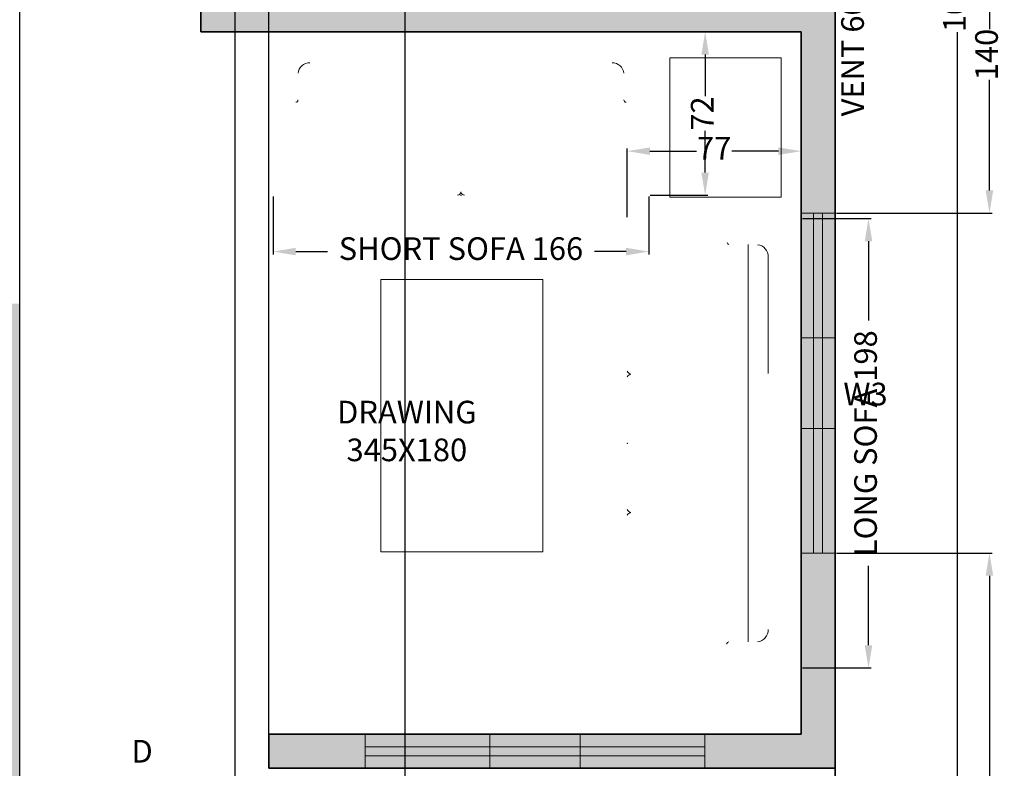
# Model space of a CAD drawing. Units: centimetres. Extents: x 2401 to 3632, y 2122 to 3526.
# Tile 6 of 10: x 2885 to 3320, y 2591 to 2921. Entities that reach past the tile are written whole.
import ezdxf

# ---------------------------------------------------------------- set-up
doc = ezdxf.new("R2010")
doc.units = ezdxf.units.CM
for name, color, linetype, lineweight in [('A-ANNO-DIMS', 9, 'Continuous', 18), ('A-ANNO-TEXT', 9, 'Continuous', 18), ('A-AREA-IDEN', 9, 'Continuous', 25), ('A-FURN', 9, 'Continuous', 18), ('A-GLAZ', 4, 'Continuous', 18), ('A-WALL', 7, 'Continuous', 35)]:
    doc.layers.add(name, color=color, linetype=linetype, lineweight=lineweight)
doc.layers.add('A-GLAZ-PATT', color=251, linetype='Continuous', lineweight=13, true_color=0x636466)
doc.layers.add('A-WALL-PATT', color=18, linetype='Continuous', lineweight=13, true_color=0x000000)
doc.styles.get("Standard").update_dxf_attribs({"font": 'arial.ttf'})
doc.dimstyles.new('ISO-25', dxfattribs={"dimtxt": 10, "dimasz": 10, "dimexe": 1.25, "dimexo": 0.625, "dimtad": 0, "dimtxsty": 'Standard', "dimcen": 2.5, "dimadec": 0, "dimazin": 0, "dimtfac": 1, "dimtmove": 0, "dimatfit": 3, "dimfxl": 1, "dimarcsym": 0})

# ---------------------------------------------------------------- blocks, each defined once
blk = doc.blocks.new('Clinicians and patient chairs 9_dwgmodels.com')
at = {"color": 0}
for points in [[(-907.9, 0, 0, 0, 0), (-959.6, -11.1, 4.62, 4.62, 0)], [(907.9, 0, 0, 0, 0), (-907.9, 0, 4.62, 4.62, 0)], [(959.6, -11.1, 0, 0, 0), (907.9, 0, 4.62, 4.62, 0)], [(-994.7, -35.9, 0, 0, 0), (-1015.6, -68.3, 4.62, 4.62, 0)], [(-959.6, -11.1, 0, 0, 0), (-994.7, -35.9, 4.62, 4.62, 0)], [(994.7, -35.9, 0, 0, 0), (959.6, -11.1, 4.62, 4.62, 0)], [(1015.6, -68.3, 0, 0, 0), (994.7, -35.9, 4.62, 4.62, 0)], [(-1015.6, -68.3, 0, 0, 0), (-1025.5, -106.3, 4.62, 4.62, 0)], [(1025.5, -106.3, 0, 0, 0), (1015.6, -68.3, 4.62, 4.62, 0)], [(-1025.5, -106.3, 0, 0, 0), (-1025.5, -779.5, 4.62, 4.62, 0)], [(1025.5, -779.5, 0, 0, 0), (1025.5, -106.3, 4.62, 4.62, 0)], [(1025.5, -779.5, 0, 0, 0), (1025.5, -117.3, 4.62, 4.62, 0)], [(-313.4, -149.9, 0, 0, 0), (-318.1, -149.9, 4.62, 4.62, 0)], [(-314.5, -150.4, 0, 0, 0), (-315.7, -159.3, 4.62, 4.62, 0)], [(-315.7, -159.3, 0, 0, 0), (-315.7, -777.3, 4.62, 4.62, 0)], [(-309.5, -148.3, 0, 0, 0), (-314.5, -150.4, 4.62, 4.62, 0)], [(-308, -148.3, 0, 0, 0), (-309.5, -148.3, 4.62, 4.62, 0)], [(-307.5, -148.3, 0, 0, 0), (-308, -148.3, 4.62, 4.62, 0)], [(242.9, -148.3, 0, 0, 0), (-307.5, -148.3, 4.62, 4.62, 0)], [(242.9, -148.3, 0, 0, 0), (296, -148.3, 4.62, 4.62, 0)], [(296, -148.3, 0, 0, 0), (307.5, -148.3, 4.62, 4.62, 0)], [(308, -148.3, 0, 0, 0), (307.5, -148.3, 4.62, 4.62, 0)], [(309.5, -148.3, 0, 0, 0), (308, -148.3, 4.62, 4.62, 0)], [(309.5, -148.3, 0, 0, 0), (314.5, -150.4, 4.62, 4.62, 0)], [(849.5, -149.9, 0, 0, 0), (313.4, -149.9, 4.62, 4.62, 0)], [(314.5, -150.4, 0, 0, 0), (315.7, -159.3, 4.62, 4.62, 0)], [(315.7, -159.3, 0, 0, 0), (315.7, -777.3, 4.62, 4.62, 0)], [(315.7, -161.8, 0, 0, 0), (315.7, -777.3, 4.62, 4.62, 0)], [(-906.6, -285, 0, 0, 0), (-906.4, -198.1, 4.62, 4.62, 0)], [(906.9, -327, 0, 0, 0), (906.4, -199.7, 4.62, 4.62, 0)], [(-906.8, -305.4, 0, 0, 0), (-906.9, -324.5, 4.62, 4.62, 0)], [(-906.6, -285, 0, 0, 0), (-906.8, -305.4, 4.62, 4.62, 0)], [(-1023, -329.7, 0, 0, 0), (-1019.2, -332.9, 4.62, 4.62, 0)], [(-1019.8, -340.2, 0, 0, 0), (-1023, -348.6, 4.62, 4.62, 0)], [(-1010.3, -335.9, 0, 0, 0), (-1019.8, -340.2, 4.62, 4.62, 0)], [(-1019.2, -332.9, 0, 0, 0), (-1019, -333, 4.62, 4.62, 0)], [(-1019, -333, 0, 0, 0), (-1018.9, -333.1, 4.62, 4.62, 0)], [(-1013.9, -334.2, 0, 0, 0), (-1018.9, -333.1, 4.62, 4.62, 0)], [(-1013.9, -334.2, 0, 0, 0), (-964.4, -335.7, 4.62, 4.62, 0)], [(-917.1, -337, 0, 0, 0), (-1010.3, -335.9, 4.62, 4.62, 0)], [(-964.4, -335.7, 0, 0, 0), (-927.1, -336.8, 4.62, 4.62, 0)], [(-906.9, -324.5, 0, 0, 0), (-906.9, -329.8, 4.62, 4.62, 0)], [(906.9, -327, 0, 0, 0), (906.9, -329.9, 4.62, 4.62, 0)], [(964.4, -335.7, 0, 0, 0), (914.9, -337.2, 4.62, 4.62, 0)], [(917.1, -339.4, 0, 0, 0), (1010.3, -338.4, 4.62, 4.62, 0)], [(1013.9, -334.2, 0, 0, 0), (964.4, -335.7, 4.62, 4.62, 0)], [(1010.3, -338.4, 0, 0, 0), (1019.8, -342.7, 4.62, 4.62, 0)], [(1013.9, -334.2, 0, 0, 0), (1018.9, -333.1, 4.62, 4.62, 0)], [(1018.9, -333.1, 0, 0, 0), (1019, -333, 4.62, 4.62, 0)], [(1019.2, -332.9, 0, 0, 0), (1019, -333, 4.62, 4.62, 0)], [(1023, -329.7, 0, 0, 0), (1019.2, -332.9, 4.62, 4.62, 0)], [(1019.8, -342.7, 0, 0, 0), (1023, -351.1, 4.62, 4.62, 0)], [(1023, -351.1, 0, 0, 0), (1022.6, -779.8, 4.62, 4.62, 0)], [(-1025.5, -779.5, 0, 0, 0), (-1022.2, -788.7, 4.62, 4.62, 0)], [(-1022.2, -788.7, 0, 0, 0), (-1021.6, -789.8, 4.62, 4.62, 0)], [(-1021.6, -789.8, 0, 0, 0), (-1020.6, -790.5, 4.62, 4.62, 0)], [(-1020.6, -790.5, 0, 0, 0), (-1013.6, -793.7, 4.62, 4.62, 0)], [(-1013.6, -793.7, 0, 0, 0), (1013.6, -793.7, 4.62, 4.62, 0)], [(1019.8, -788.8, 0, 0, 0), (1013.1, -793.7, 4.62, 4.62, 0)], [(1013.6, -793.7, 0, 0, 0), (1020.6, -790.5, 4.62, 4.62, 0)], [(1022.6, -779.8, 0, 0, 0), (1019.8, -788.8, 4.62, 4.62, 0)], [(1020.6, -790.5, 0, 0, 0), (1021.6, -789.8, 4.62, 4.62, 0)], [(1022.2, -788.7, 0, 0, 0), (1021.6, -789.8, 4.62, 4.62, 0)], [(1022.2, -788.7, 0, 0, 0), (1025.5, -779.5, 4.62, 4.62, 0)]]:
    blk.add_lwpolyline(points, format="xyseb", dxfattribs=at)
for points in [[(-849.5, -149.9), (-318.1, -149.9)], [(-906.5, -241.5), (906.5, -242.3)]]:
    blk.add_lwpolyline(points, dxfattribs=at)
for centre, radius, start, end in [((-851.7, -204.8), 54.9, 87.6679, 174.7256), ((851.7, -204.8), 54.9, 5.2744, 92.3321), ((-916.6, -326.8), 10.2, 267.5454, 342.4057), ((916.9, -329.4), 10, 182.6094, 270.795), ((-337, -773.8), 21.5, 292.115, 350.6304), ((-294.5, -773.8), 21.5, 189.3696, 247.885), ((294.5, -773.8), 21.5, 292.115, 350.6304), ((336.9, -773.8), 21.5, 189.3696, 247.885)]:
    blk.add_arc(centre, radius, start, end, dxfattribs=at)
blk.add_point((0, -793.7), dxfattribs=at)
blk = doc.blocks.new('Clinicians and patient chairs 13_dwgmodels.com')
at = {"color": 0}
for points in [[(-780.9, 0, 0, 0, 0), (-832.6, -11.1, 4.5, 4.5, 0)], [(-780.8, -0.7, 0, 0, 0), (-832.3, -11.8, 4.5, 4.5, 0)], [(-780.8, -0.7, 0, 0, 0), (-832.3, -11.8, 4.5, 4.5, 0)], [(780.9, 0, 0, 0, 0), (-780.9, 0, 4.5, 4.5, 0)], [(780.8, -0.7, 0, 0, 0), (-780.8, -0.7, 4.5, 4.5, 0)], [(780.8, -0.7, 0, 0, 0), (-780.8, -0.7, 4.5, 4.5, 0)], [(832.3, -11.8, 0, 0, 0), (780.8, -0.7, 4.5, 4.5, 0)], [(832.3, -11.8, 0, 0, 0), (780.8, -0.7, 4.5, 4.5, 0)], [(832.6, -11.1, 0, 0, 0), (780.9, 0, 4.5, 4.5, 0)], [(-867.7, -35.9, 0, 0, 0), (-888.6, -68.3, 4.5, 4.5, 0)], [(-867.1, -36.4, 0, 0, 0), (-888, -68.6, 4.5, 4.5, 0)], [(-867.1, -36.4, 0, 0, 0), (-888, -68.6, 4.5, 4.5, 0)], [(-872.1, -47.4, 0, 0, 0), (-872.1, -47.3, 4.5, 4.5, 0)], [(-832.6, -11.1, 0, 0, 0), (-867.7, -35.9, 4.5, 4.5, 0)], [(-832.3, -11.8, 0, 0, 0), (-867.1, -36.4, 4.5, 4.5, 0)], [(-832.3, -11.8, 0, 0, 0), (-867.1, -36.4, 4.5, 4.5, 0)], [(-854.1, -29.4, 0, 0, 0), (-854.1, -29.4, 4.5, 4.5, 0)], [(867.1, -36.4, 0, 0, 0), (832.3, -11.8, 4.5, 4.5, 0)], [(867.1, -36.4, 0, 0, 0), (832.3, -11.8, 4.5, 4.5, 0)], [(867.7, -35.9, 0, 0, 0), (832.6, -11.1, 4.5, 4.5, 0)], [(888, -68.6, 0, 0, 0), (867.1, -36.4, 4.5, 4.5, 0)], [(888, -68.6, 0, 0, 0), (867.1, -36.4, 4.5, 4.5, 0)], [(888.6, -68.3, 0, 0, 0), (867.7, -35.9, 4.5, 4.5, 0)], [(-888.6, -68.3, 0, 0, 0), (-898.5, -106.3, 4.5, 4.5, 0)], [(-888, -68.6, 0, 0, 0), (-897.8, -106.4, 4.5, 4.5, 0)], [(897.8, -106.4, 0, 0, 0), (888, -68.6, 4.5, 4.5, 0)], [(897.8, -106.4, 0, 0, 0), (888, -68.6, 4.5, 4.5, 0)], [(898.5, -106.3, 0, 0, 0), (888.6, -68.3, 4.5, 4.5, 0)], [(-898.5, -106.3, 0, 0, 0), (-898.5, -766.8, 4.5, 4.5, 0)], [(-897.8, -106.4, 0, 0, 0), (-897.8, -114.4, 4.5, 4.5, 0)], [(-897.8, -106.4, 0, 0, 0), (-897.8, -114.4, 4.5, 4.5, 0)], [(-897.8, -114.4, 0, 0, 0), (-897.8, -766.7, 4.5, 4.5, 0)], [(-897.8, -114.4, 0, 0, 0), (-897.8, -766.7, 4.5, 4.5, 0)], [(-897.8, -766.7, 0, 0, 0), (-897.8, -114.4, 4.5, 4.5, 0)], [(-896, -117.6, 0, 0, 0), (-896, -126.8, 4.5, 4.5, 0)], [(-896, -117.6, 0, 0, 0), (-896, -324.6, 4.5, 4.5, 0)], [(-896, -126.8, 0, 0, 0), (-896, -324.6, 4.5, 4.5, 0)], [(897.8, -114.4, 0, 0, 0), (897.8, -106.4, 4.5, 4.5, 0)], [(897.8, -114.4, 0, 0, 0), (897.8, -106.4, 4.5, 4.5, 0)], [(897.8, -766.7, 0, 0, 0), (897.8, -114.4, 4.5, 4.5, 0)], [(898.5, -766.8, 0, 0, 0), (898.5, -106.3, 4.5, 4.5, 0)], [(898.5, -766.8, 0, 0, 0), (898.5, -117.3, 4.5, 4.5, 0)], [(-22.2, -148.3, 0, 0, 0), (-722.5, -148.3, 4.5, 4.5, 0)], [(-8.3, -148.3, 0, 0, 0), (-22.2, -148.3, 4.5, 4.5, 0)], [(-8.3, -148.3, 0, 0, 0), (-7.7, -148.3, 4.5, 4.5, 0)], [(-7.7, -148.3, 0, 0, 0), (-6.2, -148.3, 4.5, 4.5, 0)], [(-6.2, -148.3, 0, 0, 0), (-1.3, -150.4, 4.5, 4.5, 0)], [(2.3, -149.9, 0, 0, 0), (-2.3, -149.9, 4.5, 4.5, 0)], [(-1.3, -150.4, 0, 0, 0), (0, -159.3, 4.5, 4.5, 0)], [(1.3, -150.4, 0, 0, 0), (0, -159.3, 4.5, 4.5, 0)], [(0, -159.3, 0, 0, 0), (0, -764.6, 4.5, 4.5, 0)], [(0, -159.3, 0, 0, 0), (0, -764.6, 4.5, 4.5, 0)], [(6.2, -148.3, 0, 0, 0), (1.3, -150.4, 4.5, 4.5, 0)], [(7.7, -148.3, 0, 0, 0), (6.2, -148.3, 4.5, 4.5, 0)], [(8.3, -148.3, 0, 0, 0), (7.7, -148.3, 4.5, 4.5, 0)], [(22.2, -148.3, 0, 0, 0), (8.3, -148.3, 4.5, 4.5, 0)], [(206.6, -148.3, 0, 0, 0), (22.2, -148.3, 4.5, 4.5, 0)], [(206.6, -148.3, 0, 0, 0), (722.5, -148.3, 4.5, 4.5, 0)], [(-779.6, -285, 0, 0, 0), (-779.4, -198.1, 4.5, 4.5, 0)], [(779.6, -285, 0, 0, 0), (779.4, -198.1, 4.5, 4.5, 0)], [(-896, -321.9, 0, 0, 0), (-896, -251.5, 4.5, 4.5, 0)], [(-896, -317.7, 0, 0, 0), (-896, -329.7, 4.5, 4.5, 0)], [(-896, -320.4, 0, 0, 0), (-896, -324.6, 4.5, 4.5, 0)], [(-896, -321.9, 0, 0, 0), (-896, -329.7, 4.5, 4.5, 0)], [(-896, -329.7, 0, 0, 0), (-896, -321.9, 4.5, 4.5, 0)], [(-896, -329.7, 0, 0, 0), (-892.2, -332.9, 4.5, 4.5, 0)], [(-779.8, -305.4, 0, 0, 0), (-779.9, -324.5, 4.5, 4.5, 0)], [(-779.6, -285, 0, 0, 0), (-779.8, -305.4, 4.5, 4.5, 0)], [(779.6, -285, 0, 0, 0), (779.8, -305.4, 4.5, 4.5, 0)], [(779.8, -305.4, 0, 0, 0), (779.9, -324.5, 4.5, 4.5, 0)], [(896, -329.7, 0, 0, 0), (892.2, -332.9, 4.5, 4.5, 0)], [(-892.2, -332.9, 0, 0, 0), (-892, -333, 4.5, 4.5, 0)], [(-892, -333, 0, 0, 0), (-891.9, -333.1, 4.5, 4.5, 0)], [(-886.9, -334.2, 0, 0, 0), (-891.9, -333.1, 4.5, 4.5, 0)], [(-886.9, -334.2, 0, 0, 0), (-837.4, -335.7, 4.5, 4.5, 0)], [(-837.4, -335.7, 0, 0, 0), (-790.1, -337, 4.5, 4.5, 0)], [(837.4, -335.7, 0, 0, 0), (790.1, -337, 4.5, 4.5, 0)], [(886.9, -334.2, 0, 0, 0), (837.4, -335.7, 4.5, 4.5, 0)], [(886.9, -334.2, 0, 0, 0), (891.9, -333.1, 4.5, 4.5, 0)], [(891.9, -333.1, 0, 0, 0), (892, -333, 4.5, 4.5, 0)], [(892.2, -332.9, 0, 0, 0), (892, -333, 4.5, 4.5, 0)], [(-898.5, -766.8, 0, 0, 0), (-895.2, -776, 4.5, 4.5, 0)], [(-895.2, -776, 0, 0, 0), (-898.5, -766.8, 4.5, 4.5, 0)], [(-897.8, -766.7, 0, 0, 0), (-894.5, -775.7, 4.5, 4.5, 0)], [(-897.8, -766.7, 0, 0, 0), (-894.5, -775.7, 4.5, 4.5, 0)], [(-894.5, -775.7, 0, 0, 0), (-897.8, -766.7, 4.5, 4.5, 0)], [(-894.5, -775.7, 0, 0, 0), (-897.8, -766.7, 4.5, 4.5, 0)], [(-895.2, -776, 0, 0, 0), (-894.6, -777.1, 4.5, 4.5, 0)], [(-894.6, -777.1, 0, 0, 0), (-895.2, -776, 4.5, 4.5, 0)], [(-894.5, -775.7, 0, 0, 0), (-894, -776.6, 4.5, 4.5, 0)], [(-894.5, -775.7, 0, 0, 0), (-894, -776.6, 4.5, 4.5, 0)], [(-894, -776.6, 0, 0, 0), (-894.5, -775.7, 4.5, 4.5, 0)], [(-894, -776.6, 0, 0, 0), (-894.5, -775.7, 4.5, 4.5, 0)], [(-894.6, -777.1, 0, 0, 0), (-893.6, -777.8, 4.5, 4.5, 0)], [(-893.6, -777.8, 0, 0, 0), (-894.6, -777.1, 4.5, 4.5, 0)], [(-894, -776.6, 0, 0, 0), (-893.2, -777.2, 4.5, 4.5, 0)], [(-894, -776.6, 0, 0, 0), (-893.2, -777.2, 4.5, 4.5, 0)], [(-893.2, -777.2, 0, 0, 0), (-894, -776.6, 4.5, 4.5, 0)], [(-893.2, -777.2, 0, 0, 0), (-894, -776.6, 4.5, 4.5, 0)], [(-893.6, -777.8, 0, 0, 0), (-886.6, -781, 4.5, 4.5, 0)], [(-886.6, -781, 0, 0, 0), (-893.6, -777.8, 4.5, 4.5, 0)], [(-893.2, -777.2, 0, 0, 0), (-886.5, -780.3, 4.5, 4.5, 0)], [(-893.2, -777.2, 0, 0, 0), (-886.5, -780.3, 4.5, 4.5, 0)], [(-886.5, -780.3, 0, 0, 0), (-893.2, -777.2, 4.5, 4.5, 0)], [(-886.5, -780.3, 0, 0, 0), (-893.2, -777.2, 4.5, 4.5, 0)], [(-886.6, -781, 0, 0, 0), (886.6, -781, 4.5, 4.5, 0)], [(886.6, -781, 0, 0, 0), (-886.6, -781, 4.5, 4.5, 0)], [(-886.5, -780.3, 0, 0, 0), (886.5, -780.3, 4.5, 4.5, 0)], [(-886.5, -780.3, 0, 0, 0), (886.5, -780.3, 4.5, 4.5, 0)], [(886.5, -780.3, 0, 0, 0), (-886.5, -780.3, 4.5, 4.5, 0)], [(886.5, -780.3, 0, 0, 0), (-886.5, -780.3, 4.5, 4.5, 0)], [(886.5, -780.3, 0, 0, 0), (893.2, -777.2, 4.5, 4.5, 0)], [(886.5, -780.3, 0, 0, 0), (893.2, -777.2, 4.5, 4.5, 0)], [(893.2, -777.2, 0, 0, 0), (886.5, -780.3, 4.5, 4.5, 0)], [(893.2, -777.2, 0, 0, 0), (886.5, -780.3, 4.5, 4.5, 0)], [(886.6, -781, 0, 0, 0), (893.6, -777.8, 4.5, 4.5, 0)], [(893.6, -777.8, 0, 0, 0), (886.6, -781, 4.5, 4.5, 0)], [(893.2, -777.2, 0, 0, 0), (894, -776.6, 4.5, 4.5, 0)], [(893.2, -777.2, 0, 0, 0), (894, -776.6, 4.5, 4.5, 0)], [(894, -776.6, 0, 0, 0), (893.2, -777.2, 4.5, 4.5, 0)], [(894, -776.6, 0, 0, 0), (893.2, -777.2, 4.5, 4.5, 0)], [(893.6, -777.8, 0, 0, 0), (894.6, -777.1, 4.5, 4.5, 0)], [(894.6, -777.1, 0, 0, 0), (893.6, -777.8, 4.5, 4.5, 0)], [(894.5, -775.7, 0, 0, 0), (894, -776.6, 4.5, 4.5, 0)], [(894.5, -775.7, 0, 0, 0), (894, -776.6, 4.5, 4.5, 0)], [(894.5, -775.7, 0, 0, 0), (894, -776.6, 4.5, 4.5, 0)], [(894.5, -775.7, 0, 0, 0), (894, -776.6, 4.5, 4.5, 0)], [(894.5, -775.7, 0, 0, 0), (897.8, -766.7, 4.5, 4.5, 0)], [(894.5, -775.7, 0, 0, 0), (897.8, -766.7, 4.5, 4.5, 0)], [(897.8, -766.7, 0, 0, 0), (894.5, -775.7, 4.5, 4.5, 0)], [(897.8, -766.7, 0, 0, 0), (894.5, -775.7, 4.5, 4.5, 0)], [(895.2, -776, 0, 0, 0), (894.6, -777.1, 4.5, 4.5, 0)], [(895.2, -776, 0, 0, 0), (894.6, -777.1, 4.5, 4.5, 0)], [(895.2, -776, 0, 0, 0), (898.5, -766.8, 4.5, 4.5, 0)], [(898.5, -766.8, 0, 0, 0), (895.2, -776, 4.5, 4.5, 0)]]:
    blk.add_lwpolyline(points, format="xyseb", dxfattribs=at)
for points in [[(-779.9, -324.5), (-779.9, -328.3)], [(779.9, -324.5), (779.9, -325.8)]]:
    blk.add_lwpolyline(points, dxfattribs=at)
for centre, radius, start, end in [((-724.7, -203.1), 54.9, 87.6679, 174.7255), ((724.7, -203.1), 54.9, 5.2744, 92.3321), ((-789.7, -327.1), 9.9, 267.955, 352.9309), ((791.8, -325.1), 12, 183.2786, 261.4861), ((-17.2, -763), 17.3, 271.1045, 354.6239), ((17.2, -763), 17.3, 185.3761, 268.8955)]:
    blk.add_arc(centre, radius, start, end, dxfattribs=at)
blk.add_point((0, -781), dxfattribs=at)
blk = doc.blocks.new('*D14')
at = {"layer": 'A-ANNO-DIMS', "color": 0, "lineweight": -2, "transparency": 16777216}
for p, q in [((3246.06, 3451.1), (3300.7, 3451.1)), ((3299.45, 3441.1), (3299.45, 2946.17)), ((3299.45, 2421.1), (3299.45, 2916.04)), ((3246.06, 2411.1), (3300.7, 2411.1))]:
    blk.add_line(p, q, dxfattribs=at)
at = {"layer": 'A-ANNO-DIMS', "color": 0, "transparency": 16777216}
for points in [[(3297.79, 3441.1), (3301.12, 3441.1), (3299.45, 3451.1)], [(3297.79, 2421.1), (3301.12, 2421.1), (3299.45, 2411.1)]]:
    blk.add_solid(points, dxfattribs=at)
at = {"layer": 'Defpoints', "color": 0, "transparency": 16777216}
for p in [(3245.44, 3451.1), (3245.44, 2411.1), (3299.45, 2411.1)]:
    blk.add_point(p, dxfattribs=at)
at = {"layer": 'A-ANNO-DIMS', "color": 0, "transparency": 16777216, "insert": (3299.45, 2931.1), "char_height": 10, "attachment_point": 5, "rotation": 90}
blk.add_mtext('1040', dxfattribs=at)
blk = doc.blocks.new('WIN-1500-3P')
for p, q in [((0, 15), (0, 0)), ((55, 15), (55, 0)), ((95, 15), (95, 0)), ((150, 15), (150, 0)), ((0, 9.5), (150, 9.5)), ((0, 5.5), (150, 5.5))]:
    blk.add_line(p, q)
blk = doc.blocks.new('*D22')
at = {"layer": 'A-ANNO-DIMS', "color": 0, "lineweight": -2, "transparency": 16777216}
for p, q in [((3246.06, 3036.1), (3255.69, 3036.1)), ((3254.44, 3026.1), (3254.44, 2986.1)), ((3246.06, 2976.1), (3255.69, 2976.1)), ((3254.44, 2976.1), (3254.44, 2966.1))]:
    blk.add_line(p, q, dxfattribs=at)
at = {"layer": 'A-ANNO-DIMS', "color": 0, "transparency": 16777216}
for points in [[(3252.77, 3026.1), (3256.1, 3026.1), (3254.44, 3036.1)], [(3252.77, 2986.1), (3256.1, 2986.1), (3254.44, 2976.1)]]:
    blk.add_solid(points, dxfattribs=at)
at = {"layer": 'Defpoints', "color": 0, "transparency": 16777216}
for p in [(3245.44, 3036.1), (3245.44, 2976.1), (3254.44, 2976.1)]:
    blk.add_point(p, dxfattribs=at)
at = {"layer": 'A-ANNO-DIMS', "color": 0, "transparency": 16777216, "insert": (3254.44, 2920.31), "char_height": 10, "attachment_point": 5, "rotation": 90}
blk.add_mtext('VENT 60 TYP.', dxfattribs=at)
blk = doc.blocks.new('*D34')
at = {"layer": 'A-ANNO-DIMS', "color": 0, "lineweight": -2, "transparency": 16777216}
for p, q in [((3231.06, 2833.71), (3261.43, 2833.71)), ((3260.18, 2823.71), (3260.18, 2788.71)), ((3260.18, 2645.39), (3260.18, 2680.4)), ((3231.06, 2635.39), (3261.43, 2635.39))]:
    blk.add_line(p, q, dxfattribs=at)
at = {"layer": 'A-ANNO-DIMS', "color": 0, "transparency": 16777216}
for points in [[(3258.52, 2823.71), (3261.85, 2823.71), (3260.18, 2833.71)], [(3258.52, 2645.39), (3261.85, 2645.39), (3260.18, 2635.39)]]:
    blk.add_solid(points, dxfattribs=at)
at = {"layer": 'Defpoints', "color": 0, "transparency": 16777216}
for p in [(3230.44, 2833.71), (3230.44, 2635.39), (3260.18, 2635.39)]:
    blk.add_point(p, dxfattribs=at)
at = {"layer": 'A-ANNO-DIMS', "color": 0, "transparency": 16777216, "insert": (3260.18, 2734.55), "char_height": 10, "attachment_point": 5, "rotation": 90}
blk.add_mtext('LONG SOFA 198', dxfattribs=at)
blk = doc.blocks.new('*D35')
at = {"layer": 'A-ANNO-DIMS', "color": 0, "lineweight": -2, "transparency": 16777216}
for p, q in [((3153.69, 2834.33), (3153.69, 2864.7)), ((3163.69, 2863.45), (3184.32, 2863.45)), ((3220.44, 2863.45), (3199.81, 2863.45)), ((3230.44, 2834.33), (3230.44, 2864.7))]:
    blk.add_line(p, q, dxfattribs=at)
at = {"layer": 'A-ANNO-DIMS', "color": 0, "transparency": 16777216}
for points in [[(3163.69, 2865.12), (3163.69, 2861.79), (3153.69, 2863.45)], [(3220.44, 2865.12), (3220.44, 2861.79), (3230.44, 2863.45)]]:
    blk.add_solid(points, dxfattribs=at)
at = {"layer": 'Defpoints', "color": 0, "transparency": 16777216}
for p in [(3230.44, 2863.45), (3153.69, 2833.71), (3230.44, 2833.71)]:
    blk.add_point(p, dxfattribs=at)
at = {"layer": 'A-ANNO-DIMS', "color": 0, "transparency": 16777216, "insert": (3192.06, 2863.45), "char_height": 10, "attachment_point": 5}
blk.add_mtext('77', dxfattribs=at)
blk = doc.blocks.new('*D36')
at = {"layer": 'A-ANNO-DIMS', "color": 0, "lineweight": -2, "transparency": 16777216}
for p, q in [((2997.33, 2843.4), (2997.33, 2817.9)), ((3163.19, 2843.4), (3163.19, 2817.9)), ((3007.33, 2819.15), (3021.27, 2819.15)), ((3153.19, 2819.15), (3139.25, 2819.15))]:
    blk.add_line(p, q, dxfattribs=at)
at = {"layer": 'A-ANNO-DIMS', "color": 0, "transparency": 16777216}
for points in [[(3007.33, 2820.81), (3007.33, 2817.48), (2997.33, 2819.15)], [(3153.19, 2820.81), (3153.19, 2817.48), (3163.19, 2819.15)]]:
    blk.add_solid(points, dxfattribs=at)
at = {"layer": 'Defpoints', "color": 0, "transparency": 16777216}
for p in [(2997.33, 2844.03), (3163.19, 2844.03), (3163.19, 2819.15)]:
    blk.add_point(p, dxfattribs=at)
at = {"layer": 'A-ANNO-DIMS', "color": 0, "transparency": 16777216, "insert": (3080.26, 2819.15), "char_height": 10, "attachment_point": 5}
blk.add_mtext('SHORT SOFA 166', dxfattribs=at)
blk = doc.blocks.new('*D37')
at = {"layer": 'A-ANNO-DIMS', "color": 0, "lineweight": -2, "transparency": 16777216}
for p, q in [((3163.82, 2916.11), (3189.32, 2916.11)), ((3188.07, 2906.11), (3188.07, 2887.76)), ((3188.07, 2854.03), (3188.07, 2872.37)), ((3163.82, 2844.03), (3189.32, 2844.03))]:
    blk.add_line(p, q, dxfattribs=at)
at = {"layer": 'A-ANNO-DIMS', "color": 0, "transparency": 16777216}
for points in [[(3186.41, 2906.11), (3189.74, 2906.11), (3188.07, 2916.11)], [(3186.41, 2854.03), (3189.74, 2854.03), (3188.07, 2844.03)]]:
    blk.add_solid(points, dxfattribs=at)
at = {"layer": 'Defpoints', "color": 0, "transparency": 16777216}
for p in [(3163.19, 2916.11), (3188.07, 2916.11), (3163.19, 2844.03)]:
    blk.add_point(p, dxfattribs=at)
at = {"layer": 'A-ANNO-DIMS', "color": 0, "transparency": 16777216, "insert": (3188.07, 2880.07), "char_height": 10, "attachment_point": 5, "rotation": 90}
blk.add_mtext('72', dxfattribs=at)
blk = doc.blocks.new('*D43')
at = {"layer": 'A-ANNO-DIMS', "color": 0, "lineweight": -2, "transparency": 16777216}
for p, q in [((3246.06, 2686.1), (3314.84, 2686.1)), ((3313.59, 2676.1), (3313.59, 2560.4)), ((3313.59, 2421.1), (3313.59, 2536.81)), ((3246.06, 2411.1), (3314.84, 2411.1))]:
    blk.add_line(p, q, dxfattribs=at)
at = {"layer": 'A-ANNO-DIMS', "color": 0, "transparency": 16777216}
for points in [[(3311.92, 2676.1), (3315.25, 2676.1), (3313.59, 2686.1)], [(3311.92, 2421.1), (3315.25, 2421.1), (3313.59, 2411.1)]]:
    blk.add_solid(points, dxfattribs=at)
at = {"layer": 'Defpoints', "color": 0, "transparency": 16777216}
for p in [(3245.44, 2686.1), (3313.59, 2686.1), (3245.44, 2411.1)]:
    blk.add_point(p, dxfattribs=at)
at = {"layer": 'A-ANNO-DIMS', "color": 0, "transparency": 16777216, "insert": (3313.59, 2548.6), "char_height": 10, "attachment_point": 5, "rotation": 90}
blk.add_mtext('275', dxfattribs=at)
blk = doc.blocks.new('*D44')
at = {"layer": 'A-ANNO-DIMS', "color": 0, "lineweight": -2, "transparency": 16777216}
for p, q in [((3246.06, 2976.1), (3314.84, 2976.1)), ((3313.59, 2966.1), (3313.59, 2917.29)), ((3313.59, 2846.1), (3313.59, 2894.92)), ((3246.06, 2836.1), (3314.84, 2836.1))]:
    blk.add_line(p, q, dxfattribs=at)
at = {"layer": 'A-ANNO-DIMS', "color": 0, "transparency": 16777216}
for points in [[(3311.92, 2966.1), (3315.25, 2966.1), (3313.59, 2976.1)], [(3311.92, 2846.1), (3315.25, 2846.1), (3313.59, 2836.1)]]:
    blk.add_solid(points, dxfattribs=at)
at = {"layer": 'Defpoints', "color": 0, "transparency": 16777216}
for p in [(3245.44, 2976.1), (3313.59, 2976.1), (3245.44, 2836.1)]:
    blk.add_point(p, dxfattribs=at)
at = {"layer": 'A-ANNO-DIMS', "color": 0, "transparency": 16777216, "insert": (3313.59, 2906.1), "char_height": 10, "attachment_point": 5, "rotation": 90}
blk.add_mtext('140', dxfattribs=at)
blk = doc.blocks.new('*D50')
at = {"layer": 'A-ANNO-DIMS', "color": 0, "lineweight": -2, "transparency": 16777216}
for p, q in [((2980.44, 3095.48), (2980.44, 2196.7)), ((3055.44, 3080.48), (3055.44, 2196.7)), ((2990.44, 2197.95), (3010.15, 2197.95)), ((3045.44, 2197.95), (3025.72, 2197.95))]:
    blk.add_line(p, q, dxfattribs=at)
at = {"layer": 'A-ANNO-DIMS', "color": 0, "transparency": 16777216}
for points in [[(2990.44, 2199.62), (2990.44, 2196.29), (2980.44, 2197.95)], [(3045.44, 2199.62), (3045.44, 2196.29), (3055.44, 2197.95)]]:
    blk.add_solid(points, dxfattribs=at)
at = {"layer": 'Defpoints', "color": 0, "transparency": 16777216}
for p in [(2980.44, 3096.1), (3055.44, 3081.1), (3055.44, 2197.95)]:
    blk.add_point(p, dxfattribs=at)
at = {"layer": 'A-ANNO-DIMS', "color": 0, "transparency": 16777216, "insert": (3017.94, 2197.95), "char_height": 10, "attachment_point": 5}
blk.add_mtext('75', dxfattribs=at)
blk = doc.blocks.new('*D52')
at = {"layer": 'A-ANNO-DIMS', "color": 0, "lineweight": -2, "transparency": 16777216}
for p, q in [((2885.44, 2411.73), (2885.44, 3520.5)), ((2895.44, 3519.25), (2929.25, 3519.25)), ((2985.44, 3519.25), (2951.62, 3519.25)), ((2995.44, 2591.73), (2995.44, 3520.5))]:
    blk.add_line(p, q, dxfattribs=at)
at = {"layer": 'A-ANNO-DIMS', "color": 0, "transparency": 16777216}
for points in [[(2895.44, 3520.92), (2895.44, 3517.59), (2885.44, 3519.25)], [(2985.44, 3520.92), (2985.44, 3517.59), (2995.44, 3519.25)]]:
    blk.add_solid(points, dxfattribs=at)
at = {"layer": 'Defpoints', "color": 0, "transparency": 16777216}
for p in [(2995.44, 3519.25), (2995.44, 2591.1), (2885.44, 2411.1)]:
    blk.add_point(p, dxfattribs=at)
at = {"layer": 'A-ANNO-DIMS', "color": 0, "transparency": 16777216, "insert": (2940.44, 3519.25), "char_height": 10, "attachment_point": 5}
blk.add_mtext('110', dxfattribs=at)

msp = doc.modelspace()

# ---------------------------------------------------------------- hatches: boundary and pattern name
at = {"layer": 'A-GLAZ-PATT'}
h = msp.add_hatch(color=256, dxfattribs=at)
h.dxf.hatch_style = 1
h.paths.add_polyline_path([(2505.936, 3356.104), (2500.436, 3356.104), (2500.436, 3301.104), (2505.936, 3301.104)])
h.paths.add_polyline_path([(2509.936, 3356.104), (2505.936, 3356.104), (2505.936, 3301.104), (2509.936, 3301.104)])
h.paths.add_polyline_path([(2515.436, 3335.674), (2515.436, 3356.104), (2509.936, 3356.104), (2509.936, 3301.104), (2515.436, 3301.104)])
h.paths.add_polyline_path([(2509.936, 3301.104), (2505.936, 3301.104), (2505.936, 3261.104), (2509.936, 3261.104)])
h.paths.add_polyline_path([(2515.436, 3301.104), (2509.936, 3301.104), (2509.936, 3261.104), (2515.436, 3261.104)])
h.paths.add_polyline_path([(2505.936, 3301.104), (2500.436, 3301.104), (2500.436, 3261.104), (2505.936, 3261.104)])
h.paths.add_polyline_path([(2515.436, 3261.104), (2509.936, 3261.104), (2509.936, 3206.104), (2515.436, 3206.104)])
h.paths.add_polyline_path([(2505.936, 3261.104), (2500.436, 3261.104), (2500.436, 3206.104), (2505.936, 3206.104)])
h.paths.add_polyline_path([(2509.936, 3261.104), (2505.936, 3261.104), (2505.936, 3206.104), (2509.936, 3206.104)])
h.paths.add_polyline_path([(3127.936, 3451.104), (3072.936, 3451.104), (3072.936, 3445.604), (3127.936, 3445.604)])
h.paths.add_polyline_path([(3032.936, 3441.604), (2977.936, 3441.604), (2977.936, 3436.104), (3032.936, 3436.104)])
h.paths.add_polyline_path([(3032.936, 3451.104), (2977.936, 3451.104), (2977.936, 3445.604), (3032.936, 3445.604)])
h.paths.add_polyline_path([(3032.936, 3445.604), (2977.936, 3445.604), (2977.936, 3441.604), (3032.936, 3441.604)])
h.paths.add_polyline_path([(3072.936, 3451.104), (3032.936, 3451.104), (3032.936, 3445.604), (3072.936, 3445.604)])
h.paths.add_polyline_path([(3072.936, 3445.604), (3032.936, 3445.604), (3032.936, 3441.604), (3072.936, 3441.604)])
h.paths.add_polyline_path([(3072.936, 3441.604), (3032.936, 3441.604), (3032.936, 3436.104), (3072.936, 3436.104)])
h.paths.add_polyline_path([(3127.936, 3441.604), (3072.936, 3441.604), (3072.936, 3436.104), (3127.936, 3436.104)])
h.paths.add_polyline_path([(3127.936, 3445.604), (3072.936, 3445.604), (3072.936, 3441.604), (3127.936, 3441.604)])
h.paths.add_polyline_path([(3245.436, 3356.104), (3239.936, 3356.104), (3239.936, 3301.104), (3245.436, 3301.104)])
h.paths.add_polyline_path([(3239.936, 3356.104), (3235.936, 3356.104), (3235.936, 3301.104), (3239.936, 3301.104)])
h.paths.add_polyline_path([(3235.936, 3356.104), (3230.436, 3356.104), (3230.436, 3301.104), (3235.936, 3301.104)])
h.paths.add_polyline_path([(3235.936, 3301.104), (3230.436, 3301.104), (3230.436, 3261.104), (3235.936, 3261.104)])
h.paths.add_polyline_path([(3239.936, 3301.104), (3235.936, 3301.104), (3235.936, 3261.104), (3239.936, 3261.104)])
h.paths.add_polyline_path([(3245.436, 3301.104), (3239.936, 3301.104), (3239.936, 3261.104), (3245.436, 3261.104)])
h.paths.add_polyline_path([(3245.436, 3261.104), (3239.936, 3261.104), (3239.936, 3206.104), (3245.436, 3206.104)])
h.paths.add_polyline_path([(3239.936, 3261.104), (3235.936, 3261.104), (3235.936, 3206.104), (3239.936, 3206.104)])
h.paths.add_polyline_path([(3235.936, 3261.104), (3230.436, 3261.104), (3230.436, 3206.104), (3235.936, 3206.104)])
h.paths.add_polyline_path([(3239.936, 3036.104), (3235.936, 3036.104), (3235.936, 2976.104), (3239.936, 2976.104)])
h.paths.add_polyline_path([(3235.936, 3036.104), (3230.436, 3036.104), (3230.436, 2976.104), (3235.936, 2976.104)])
h.paths.add_polyline_path([(3245.436, 3036.104), (3239.936, 3036.104), (3239.936, 2976.104), (3245.436, 2976.104)])
h.paths.add_polyline_path([(3235.936, 2836.104), (3230.436, 2836.104), (3230.436, 2781.104), (3235.936, 2781.104)])
h.paths.add_polyline_path([(3245.436, 2836.104), (3239.936, 2836.104), (3239.936, 2781.104), (3245.436, 2781.104)])
h.paths.add_polyline_path([(3239.936, 2836.104), (3235.936, 2836.104), (3235.936, 2781.104), (3239.936, 2781.104)])
h.paths.add_polyline_path([(3245.436, 2781.104), (3239.936, 2781.104), (3239.936, 2741.104), (3245.436, 2741.104)])
h.paths.add_polyline_path([(3239.936, 2781.104), (3235.936, 2781.104), (3235.936, 2741.104), (3239.936, 2741.104)])
h.paths.add_polyline_path([(3235.936, 2781.104), (3230.436, 2781.104), (3230.436, 2741.104), (3235.936, 2741.104)])
h.paths.add_polyline_path([(3245.436, 2741.104), (3239.936, 2741.104), (3239.936, 2686.104), (3245.436, 2686.104)])
h.paths.add_polyline_path([(3239.936, 2741.104), (3235.936, 2741.104), (3235.936, 2686.104), (3239.936, 2686.104)])
h.paths.add_polyline_path([(3235.936, 2741.104), (3230.436, 2741.104), (3230.436, 2686.104), (3235.936, 2686.104)])
h.paths.add_polyline_path([(3187.936, 2606.104), (3132.936, 2606.104), (3132.936, 2600.604), (3187.936, 2600.604)])
h.paths.add_polyline_path([(3187.936, 2600.604), (3132.936, 2600.604), (3132.936, 2596.604), (3187.936, 2596.604)])
h.paths.add_polyline_path([(3187.936, 2596.604), (3132.936, 2596.604), (3132.936, 2591.104), (3187.936, 2591.104)])
h.paths.add_polyline_path([(3132.936, 2596.604), (3092.936, 2596.604), (3092.936, 2591.104), (3132.936, 2591.104)])
h.paths.add_polyline_path([(3132.936, 2600.604), (3092.936, 2600.604), (3092.936, 2596.604), (3132.936, 2596.604)])
h.paths.add_polyline_path([(3132.936, 2606.104), (3092.936, 2606.104), (3092.936, 2600.604), (3132.936, 2600.604)])
h.paths.add_polyline_path([(3092.936, 2596.604), (3037.936, 2596.604), (3037.936, 2591.104), (3092.936, 2591.104)])
h.paths.add_polyline_path([(3092.936, 2600.604), (3037.936, 2600.604), (3037.936, 2596.604), (3092.936, 2596.604)])
h.paths.add_polyline_path([(3092.936, 2606.104), (3037.936, 2606.104), (3037.936, 2600.604), (3092.936, 2600.604)])
h.paths.add_polyline_path([(2803.613, 3432.66), (2826.471, 3432.66), (2826.471, 3453.267), (2803.613, 3453.267)], flags=9)
h.paths.add_polyline_path([(2904.038, 3087.418), (2926.896, 3087.418), (2926.896, 3108.025), (2904.038, 3108.025)], flags=9)
h.paths.add_polyline_path([(2801.908, 3105.391), (2824.766, 3105.391), (2824.766, 3125.998), (2801.908, 3125.998)], flags=9)
h.paths.add_polyline_path([(2757.576, 2660.284), (2780.434, 2660.284), (2780.434, 2680.892), (2757.576, 2680.892)], flags=9)
h.paths.add_polyline_path([(3004.446, 3080.825), (3027.304, 3080.825), (3027.304, 3101.432), (3004.446, 3101.432)], flags=9)
h.paths.add_polyline_path([(2805.63, 2777.019), (2828.489, 2777.019), (2828.489, 2797.626), (2805.63, 2797.626)], flags=9)
h.paths.add_polyline_path([(3094.334, 2572.754), (3128.823, 2572.754), (3128.823, 2593.361), (3094.334, 2593.361)], flags=9)
h.paths.add_polyline_path([(2931.792, 2588.154), (2946.88, 2588.154), (2946.88, 2608.761), (2931.792, 2608.761)], flags=9)
h.paths.add_polyline_path([(2582.951, 2415.87), (2664.015, 2415.87), (2664.015, 2453.184), (2582.951, 2453.184)], flags=9)
h.paths.add_polyline_path([(2622.234, 2685.113), (2683.168, 2685.113), (2683.168, 2722.427), (2622.234, 2722.427)], flags=9)
h.paths.add_polyline_path([(3027.646, 2511.408), (3088.58, 2511.408), (3088.58, 2548.722), (3027.646, 2548.722)], flags=9)
h.paths.add_polyline_path([(3020.004, 2720.966), (3092.521, 2720.966), (3092.521, 2758.281), (3020.004, 2758.281)], flags=9)
h.paths.add_polyline_path([(2628.506, 2930.416), (2689.441, 2930.416), (2689.441, 2967.73), (2628.506, 2967.73)], flags=9)
h.paths.add_polyline_path([(3056.573, 2986.666), (3117.507, 2986.666), (3117.507, 3023.981), (3056.573, 3023.981)], flags=9)
h.paths.add_polyline_path([(3083.425, 3281.357), (3164.489, 3281.357), (3164.489, 3318.672), (3083.425, 3318.672)], flags=9)
h.paths.add_polyline_path([(2658.367, 3249.15), (2724.683, 3249.15), (2724.683, 3286.465), (2658.367, 3286.465)], flags=9)
h = msp.add_hatch(color=256, dxfattribs=at)
h.dxf.hatch_style = 1
h.paths.add_polyline_path([(3132.936, 2596.604), (3092.936, 2596.604), (3092.936, 2591.104), (3132.936, 2591.104)])
h.paths.add_polyline_path([(2762.936, 2281.104), (2707.936, 2281.104), (2707.936, 2275.604), (2762.936, 2275.604)])
h.paths.add_polyline_path([(2707.936, 2271.604), (2667.936, 2271.604), (2667.936, 2266.104), (2707.936, 2266.104)])
h.paths.add_polyline_path([(2762.936, 2275.604), (2707.936, 2275.604), (2707.936, 2271.604), (2762.936, 2271.604)])
h.paths.add_polyline_path([(2762.936, 2271.604), (2707.936, 2271.604), (2707.936, 2266.104), (2762.936, 2266.104)])
h.paths.add_polyline_path([(2707.936, 2275.604), (2667.936, 2275.604), (2667.936, 2271.604), (2707.936, 2271.604)])
h.paths.add_polyline_path([(2707.936, 2281.104), (2667.936, 2281.104), (2667.936, 2275.604), (2707.936, 2275.604)])
h.paths.add_polyline_path([(2667.936, 2281.104), (2612.936, 2281.104), (2612.936, 2275.604), (2667.936, 2275.604)])
h.paths.add_polyline_path([(2667.936, 2275.604), (2612.936, 2275.604), (2612.936, 2271.604), (2667.936, 2271.604)])
h.paths.add_polyline_path([(2667.936, 2271.604), (2612.936, 2271.604), (2612.936, 2266.104), (2667.936, 2266.104)])
h.paths.add_polyline_path([(2515.436, 2523.604), (2509.936, 2523.604), (2509.936, 2468.604), (2515.436, 2468.604)])
h.paths.add_polyline_path([(2509.936, 2523.604), (2505.936, 2523.604), (2505.936, 2468.604), (2509.936, 2468.604)])
h.paths.add_polyline_path([(2505.936, 2523.604), (2500.436, 2523.604), (2500.436, 2468.604), (2505.936, 2468.604)])
h.paths.add_polyline_path([(2505.936, 2468.604), (2500.436, 2468.604), (2500.436, 2428.604), (2505.936, 2428.604)])
h.paths.add_polyline_path([(2509.936, 2468.604), (2505.936, 2468.604), (2505.936, 2428.604), (2509.936, 2428.604)])
h.paths.add_polyline_path([(2515.436, 2468.604), (2509.936, 2468.604), (2509.936, 2428.604), (2515.436, 2428.604)])
h.paths.add_polyline_path([(2515.436, 2428.604), (2509.936, 2428.604), (2509.936, 2373.604), (2515.436, 2373.604)])
h.paths.add_polyline_path([(2509.936, 2428.604), (2505.936, 2428.604), (2505.936, 2373.604), (2509.936, 2373.604)])
h.paths.add_polyline_path([(2505.936, 2428.604), (2500.436, 2428.604), (2500.436, 2373.604), (2505.936, 2373.604)])
h.paths.add_polyline_path([(2505.936, 3028.604), (2500.436, 3028.604), (2500.436, 2973.604), (2505.936, 2973.604)])
h.paths.add_polyline_path([(2515.436, 3028.604), (2509.936, 3028.604), (2509.936, 2973.604), (2515.436, 2973.604)])
h.paths.add_polyline_path([(2509.936, 3028.604), (2505.936, 3028.604), (2505.936, 2973.604), (2509.936, 2973.604)])
h.paths.add_polyline_path([(2515.436, 2973.604), (2509.936, 2973.604), (2509.936, 2933.604), (2515.436, 2933.604)])
h.paths.add_polyline_path([(2509.936, 2973.604), (2505.936, 2973.604), (2505.936, 2933.604), (2509.936, 2933.604)])
h.paths.add_polyline_path([(2505.936, 2973.604), (2500.436, 2973.604), (2500.436, 2933.604), (2505.936, 2933.604)])
h.paths.add_polyline_path([(2505.936, 2933.604), (2500.436, 2933.604), (2500.436, 2878.604), (2505.936, 2878.604)])
h.paths.add_polyline_path([(2515.436, 2933.604), (2509.936, 2933.604), (2509.936, 2878.604), (2515.436, 2878.604)])
h.paths.add_polyline_path([(2509.936, 2933.604), (2505.936, 2933.604), (2505.936, 2878.604), (2509.936, 2878.604)])
at = {"layer": 'A-WALL-PATT'}
h = msp.add_hatch(color=256, dxfattribs=at)
h.dxf.hatch_style = 1
h.paths.add_polyline_path([(2765.436, 3451.104), (2500.436, 3451.104), (2500.436, 3356.104), (2515.436, 3356.104), (2515.436, 3436.104), (2765.436, 3436.104)])
h.paths.add_polyline_path([(3245.436, 3451.104), (3127.936, 3451.104), (3127.936, 3436.104), (3185.226, 3436.104), (3185.226, 3436.735), (3230.436, 3436.735), (3230.436, 3356.104), (3245.436, 3356.104)])
h.paths.add_polyline_path([(3245.436, 2686.104), (3230.436, 2686.104), (3230.436, 2606.104), (3187.936, 2606.104), (3187.936, 2591.104), (3245.436, 2591.104)])
h.paths.add_polyline_path([(3037.936, 2606.104), (2995.436, 2606.104), (2995.436, 2591.104), (3037.936, 2591.104)])
h.paths.add_polyline_path([(3245.436, 2976.104), (3230.436, 2976.104), (3230.436, 2931.104), (2980.436, 2931.104), (2980.436, 3096.104), (2965.436, 3096.104), (2965.436, 2916.104), (3230.436, 2916.104), (3230.436, 2836.104), (3245.436, 2836.104)])
h.paths.add_polyline_path([(3230.436, 3096.104), (3055.436, 3096.104), (3055.436, 3081.104), (3230.436, 3081.104)], flags=17)
h.paths.add_polyline_path([(2977.936, 3451.104), (2860.436, 3451.104), (2860.436, 3096.104), (2875.436, 3096.104), (2875.436, 3436.104), (2977.936, 3436.104)])
h.paths.add_polyline_path([(2765.436, 3126.104), (2515.436, 3126.104), (2515.436, 3206.104), (2500.436, 3206.104), (2500.436, 3028.604), (2515.436, 3028.604), (2515.436, 3111.104), (2765.436, 3111.104)])
h.paths.add_polyline_path([(2780.436, 2796.104), (2515.436, 2796.104), (2515.436, 2878.604), (2500.436, 2878.604), (2500.436, 2736.104), (2515.436, 2736.104), (2515.436, 2781.104), (2765.436, 2781.104), (2765.436, 2706.104), (2780.436, 2706.104)])
h.paths.add_polyline_path([(2780.436, 2631.104), (2515.436, 2631.104), (2515.436, 2676.104), (2500.436, 2676.104), (2500.436, 2523.604), (2515.436, 2523.604), (2515.436, 2616.104), (2780.436, 2616.104)])
h.paths.add_polyline_path([(2885.436, 2796.104), (2870.436, 2796.104), (2870.436, 2281.104), (2762.936, 2281.104), (2762.936, 2266.104), (2885.436, 2266.104)])
h.paths.add_polyline_path([(2612.936, 2281.104), (2515.436, 2281.104), (2515.436, 2373.604), (2500.436, 2373.604), (2500.436, 2266.104), (2612.936, 2266.104)])

# ---------------------------------------------------------------- linework, layer by layer
at = {"layer": 'A-FURN'}
for points in [[(3172.432, 2904.691), (3221.623, 2904.691), (3221.623, 2843.134), (3172.432, 2843.134)], [(3116.391, 2806.868), (3044.833, 2806.868), (3044.833, 2686.687), (3116.391, 2686.687)]]:
    msp.add_lwpolyline(points, close=True, dxfattribs=at)
at = {"layer": 'A-WALL'}
for p, q in [((2965.436, 2916.104), (2965.436, 3096.104)), ((3230.436, 2916.104), (2965.436, 2916.104)), ((3230.436, 2606.104), (3230.436, 2916.104)), ((3230.436, 2606.104), (2995.436, 2606.104)), ((2995.436, 2606.104), (2995.436, 2591.104)), ((3245.436, 2591.104), (2995.436, 2591.104))]:
    msp.add_line(p, q, dxfattribs=at)
msp.add_lwpolyline([(2885.436, 2411.104), (3245.436, 2411.104), (3245.436, 3451.104), (2860.436, 3451.104)], dxfattribs=at)

# ---------------------------------------------------------------- block references
at = {"layer": 'A-FURN', "xscale": 0.0922986845926026, "yscale": 0.0922986845926026, "zscale": 0.0922986845926026}
msp.add_blockref('Clinicians and patient chairs 13_dwgmodels.com', (3080.26, 2916.114), dxfattribs=at)
at = {"layer": 'A-FURN', "xscale": 0.0966898092323781, "yscale": 0.0966898092323781, "zscale": 0.0966898092323781, "rotation": 270}
msp.add_blockref('Clinicians and patient chairs 9_dwgmodels.com', (3230.436, 2734.55), dxfattribs=at)
at = {"layer": 'A-GLAZ', "rotation": 90.00000000000028}
msp.add_blockref('WIN-1500-3P', (3245.436, 2686.104), dxfattribs=at)
at = {"layer": 'A-GLAZ'}
msp.add_blockref('WIN-1500-3P', (3037.936, 2591.104), dxfattribs=at)

# ---------------------------------------------------------------- texts
at = {"layer": 'A-ANNO-TEXT', "char_height": 10, "attachment_point": 1}
for s, insert in [('\\pxqc;W3', (3225.714, 2761.264)), ('\\pxqc;D', (2906.36, 2603.614))]:
    msp.add_mtext_dynamic_manual_height_columns(s, width=66.28614, gutter_width=12.5, heights=[0], dxfattribs=dict(at, insert=insert))
at = {"layer": 'A-AREA-IDEN', "insert": (3023.222, 2753.305), "char_height": 10, "attachment_point": 1}
msp.add_mtext_dynamic_manual_height_columns('\\pxqc;DRAWING\\P345X180', width=66.28614, gutter_width=12.5, heights=[0], dxfattribs=at)

# ---------------------------------------------------------------- dimensions: what is measured, and where the dimension line sits
at = {"layer": 'A-ANNO-DIMS'}
for base, p1, p2, picture, middle in [((2995.436, 3519.254), (2885.436, 2411.104), (2995.436, 2591.104), '*D52', (2940.436, 3519.254)), ((3055.436, 2197.954), (2980.436, 3096.104), (3055.436, 3081.104), '*D50', (3017.936, 2197.954)), ((3230.436, 2863.455), (3153.69, 2833.707), (3230.436, 2833.707), '*D35', (3192.063, 2863.455))]:
    dim = msp.add_linear_dim(base=base, p1=p1, p2=p2, dimstyle='ISO-25', override={"dimdec": 0, "dimlfac": 1, "dimrnd": 0, "dimzin": 0, "dimdsep": 46, "dimlunit": 2}, dxfattribs=at)
    dim.commit()
    dim.dimension.update_dxf_attribs({"geometry": picture, "text_midpoint": middle})
for base, p1, p2, override, picture, middle in [((3299.454, 2411.104), (3245.436, 3451.104), (3245.436, 2411.104), {"dimclrd": 0, "dimclre": 0, "dimclrt": 0}, '*D14', (3299.454, 2931.104)), ((3313.586, 2976.104), (3245.436, 2836.104), (3245.436, 2976.104), {"dimdec": 0, "dimlfac": 1, "dimrnd": 0, "dimzin": 0, "dimdsep": 46, "dimlunit": 2}, '*D44', (3313.586, 2906.104)), ((3188.072, 2916.114), (3163.193, 2844.025), (3163.193, 2916.114), {"dimdec": 0, "dimlfac": 1, "dimrnd": 0, "dimzin": 0, "dimdsep": 46, "dimlunit": 2}, '*D37', (3188.072, 2880.07)), ((3313.586, 2686.104), (3245.436, 2411.104), (3245.436, 2686.104), {"dimdec": 0, "dimlfac": 1, "dimrnd": 0, "dimzin": 0, "dimdsep": 46, "dimlunit": 2}, '*D43', (3313.586, 2548.604))]:
    dim = msp.add_linear_dim(base=base, p1=p1, p2=p2, angle=90, dimstyle='ISO-25', override=override, dxfattribs=at)
    dim.commit()
    dim.dimension.update_dxf_attribs({"geometry": picture, "text_midpoint": middle})
for base, p1, p2, text, picture, middle in [((3254.436, 2976.104), (3245.436, 3036.104), (3245.436, 2976.104), 'VENT <> TYP.', '*D22', (3254.436, 2920.312)), ((3260.183, 2635.393), (3230.436, 2833.707), (3230.436, 2635.393), 'LONG SOFA <>', '*D34', (3260.183, 2734.55))]:
    dim = msp.add_linear_dim(base=base, p1=p1, p2=p2, angle=270, text=text, dimstyle='ISO-25', override={"dimdec": 0, "dimlfac": 1, "dimrnd": 0, "dimzin": 0, "dimdsep": 46, "dimlunit": 2}, dxfattribs=at)
    dim.commit()
    dim.dimension.update_dxf_attribs({"geometry": picture, "text_midpoint": middle})
dim = msp.add_linear_dim(base=(3163.193, 2819.146), p1=(2997.328, 2844.025), p2=(3163.193, 2844.025), text='SHORT SOFA <>', dimstyle='ISO-25', override={"dimdec": 0, "dimlfac": 1, "dimrnd": 0, "dimzin": 0, "dimdsep": 46, "dimlunit": 2}, dxfattribs=at)
dim.commit()
dim.dimension.update_dxf_attribs({"geometry": '*D36', "text_midpoint": (3080.26, 2819.146)})

doc.saveas('drawing.dxf')
